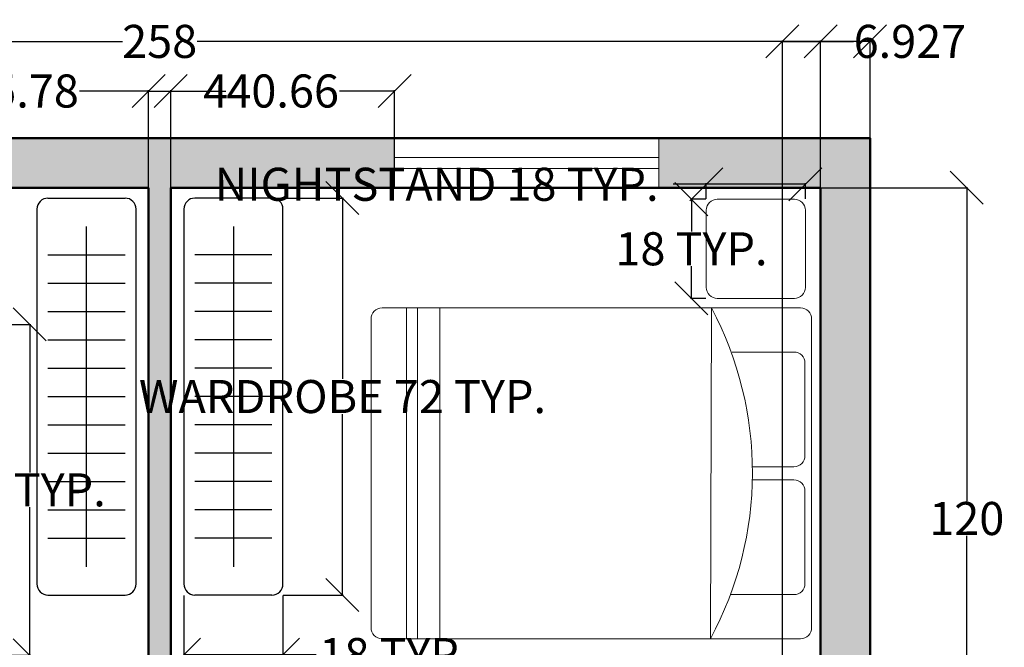
# Model space of a CAD drawing. Units: inches. Extents: x -29 to 284, y -310 to 51.
# Tile 4 of 4: x 105 to 283, y -63 to 51. Entities that reach past the tile are written whole.
import ezdxf

# ---------------------------------------------------------------- set-up
doc = ezdxf.new("R2010")
doc.units = ezdxf.units.IN
doc.header["$MEASUREMENT"] = 0
for name, color, linetype, lineweight in [('A-ANNO-DIMS', 2, 'Continuous', 18), ('A-FLOR-CASE', 9, 'Continuous', 25), ('A-FURN', 8, 'Continuous', 18), ('A-GLAZ', 4, 'Continuous', 18), ('A-WALL', 7, 'Continuous', 50)]:
    doc.layers.add(name, color=color, linetype=linetype, lineweight=lineweight)
doc.layers.add('A-WALL-PATT', color=18, linetype='Continuous', lineweight=13, true_color=0x000000)
doc.styles.get("Standard").update_dxf_attribs({"font": 'arial.ttf'})
doc.dimstyles.get("Standard").update_dxf_attribs({"dimtxt": 6, "dimasz": 6, "dimexe": 0.18, "dimexo": 0.0625, "dimgap": 0.09, "dimtad": 0, "dimtih": 1, "dimtoh": 1, "dimdec": 0, "dimzin": 0, "dimdsep": 46, "dimlunit": 4, "dimtxsty": 'Standard', "dimblk": 'OBLIQUE', "dimcen": 0.09, "dimadec": 0, "dimazin": 0, "dimtfac": 1, "dimtdec": 0, "dimtofl": 0, "dimtmove": 0, "dimatfit": 3, "dimldrblk": 'OBLIQUE', "dimfxl": 1, "dimtolj": 1, "dimtzin": 0, "dimarcsym": 0})

# ---------------------------------------------------------------- blocks, each defined once
blk = doc.blocks.new('Bed - Queen')
for p, q in [((2, 0), (58, 0)), ((10, -1.2), (26.8, -1.2)), ((33.2, -1.2), (50, -1.2)), ((0, -78), (0, -2)), ((8, -14.4), (8, -3.2)), ((28.8, -3.2), (28.8, -10.75)), ((31.2, -10.81), (31.2, -3.2)), ((52, -3.2), (52, -14.74)), ((60, -2), (60, -78)), ((0, -18.19), (60, -18.37)), ((0, -67.53), (60, -67.53)), ((0, -71.53), (60, -71.53)), ((0, -73.53), (60, -73.53)), ((58, -80), (2, -80))]:
    blk.add_line(p, q)
for centre, radius, start, end in [((2, -2), 2, 90, 180), ((58, -2), 2, 0, 90), ((10, -3.2), 2, 90, 180), ((26.8, -3.2), 2, 0, 90), ((33.2, -3.2), 2, 90, 180), ((50, -3.2), 2, 0, 90), ((29.83, -74.22), 63.48, 61.626, 118.0335), ((2, -78), 2, 180, 270), ((58, -78), 2, 270, 0)]:
    blk.add_arc(centre, radius, start, end)
blk = doc.blocks.new('WIN-48IN')
for p, q in [((0, 5.5), (48, 5.5)), ((0, 3.5), (48, 3.5))]:
    blk.add_line(p, q)
for points in [[(0, 0), (0, 9)], [(48, 9), (48, 0)]]:
    blk.add_lwpolyline(points)
blk = doc.blocks.new('WARDROBE-72IN')
for p, q in [((16, 72), (2, 72)), ((0, 70), (0, 2)), ((18, 2), (18, 70)), ((9, 66.86), (9, 5.14)), ((16, 61.71), (2, 61.71)), ((16, 56.57), (2, 56.57)), ((16, 51.43), (2, 51.43)), ((16, 46.29), (2, 46.29)), ((16, 41.14), (2, 41.14)), ((16, 36), (2, 36)), ((16, 30.86), (2, 30.86)), ((16, 25.71), (2, 25.71)), ((16, 20.57), (2, 20.57)), ((16, 15.43), (2, 15.43)), ((16, 10.29), (2, 10.29)), ((16, 0), (2, 0))]:
    blk.add_line(p, q)
for centre, start, end in [((2, 70), 90, 180), ((16, 70), 0, 90), ((2, 2), 180, 270), ((16, 2), 270, 0)]:
    blk.add_arc(centre, 2, start, end)
blk = doc.blocks.new('NIGHTSTAND-18IN')
blk.add_lwpolyline([(0, 2), (0, 16, -0.414214), (2, 18), (16, 18, -0.414214), (18, 16), (18, 2, -0.414214), (16, 0), (2, 0, -0.414214)], format="xyb", close=True)
blk = doc.blocks.new('_Oblique')
at = {"color": 0, "linetype": 'ByBlock', "lineweight": -2}
blk.add_line((-0.5, -0.5), (0.5, 0.5), dxfattribs=at)
blk = doc.blocks.new('*D23')
at = {"layer": 'A-ANNO-DIMS', "color": 0, "lineweight": -2, "transparency": 16777216}
for p, q in [((229.24, 21.07), (223.24, 21.07)), ((229.24, 18.43), (229.24, 21.25)), ((247.24, 21.07), (229.24, 21.07)), ((247.24, 18.43), (247.24, 21.25))]:
    blk.add_line(p, q, dxfattribs=at)
at = {"layer": 'Defpoints', "color": 0, "transparency": 16777216}
for p in [(229.24, 21.07), (229.24, 18.37), (247.24, 18.37)]:
    blk.add_point(p, dxfattribs=at)
at = {"layer": 'A-ANNO-DIMS', "color": 0, "lineweight": -2, "transparency": 16777216, "xscale": 6, "yscale": 6, "zscale": 6, "rotation": 180}
blk.add_blockref('_Oblique', (229.24, 21.07), dxfattribs=at)
at = {"layer": 'A-ANNO-DIMS', "color": 0, "lineweight": -2, "transparency": 16777216, "xscale": 6, "yscale": 6, "zscale": 6}
blk.add_blockref('_Oblique', (247.24, 21.07), dxfattribs=at)
at = {"layer": 'A-ANNO-DIMS', "color": 0, "transparency": 16777216, "insert": (180.28, 21.07), "char_height": 6, "attachment_point": 5}
blk.add_mtext('\\A1;NIGHTSTAND 18 TYP.', dxfattribs=at)
blk = doc.blocks.new('*D24')
at = {"layer": 'A-ANNO-DIMS', "color": 0, "lineweight": -2, "transparency": 16777216}
for p, q in [((229.17, 18.37), (226.36, 18.37)), ((226.54, 18.37), (226.54, 12.52)), ((226.54, 0.37), (226.54, 6.21)), ((229.17, 0.37), (226.36, 0.37))]:
    blk.add_line(p, q, dxfattribs=at)
at = {"layer": 'Defpoints', "color": 0, "transparency": 16777216}
for p in [(229.24, 18.37), (226.54, 0.37), (229.24, 0.37)]:
    blk.add_point(p, dxfattribs=at)
at = {"layer": 'A-ANNO-DIMS', "color": 0, "lineweight": -2, "transparency": 16777216, "xscale": 6, "yscale": 6, "zscale": 6}
for p, rotation in [((226.54, 18.37), 90), ((226.54, 0.37), 270)]:
    blk.add_blockref('_Oblique', p, dxfattribs=dict(at, rotation=rotation))
at = {"layer": 'A-ANNO-DIMS', "color": 0, "transparency": 16777216, "insert": (226.54, 9.37), "char_height": 6, "attachment_point": 5}
blk.add_mtext('\\A1;18 TYP.', dxfattribs=at)
blk = doc.blocks.new('*D26')
at = {"layer": 'A-ANNO-DIMS', "color": 0, "lineweight": -2, "transparency": 16777216}
for p, q in [((94.44, -4.36), (106.56, -4.36)), ((106.38, -4.36), (106.38, -31.2)), ((106.38, -64.36), (106.38, -37.51)), ((94.44, -64.36), (106.56, -64.36))]:
    blk.add_line(p, q, dxfattribs=at)
at = {"layer": 'Defpoints', "color": 0, "transparency": 16777216}
for p in [(94.38, -4.36), (106.38, -4.36), (94.38, -64.36)]:
    blk.add_point(p, dxfattribs=at)
at = {"layer": 'A-ANNO-DIMS', "color": 0, "lineweight": -2, "transparency": 16777216, "xscale": 6, "yscale": 6, "zscale": 6}
for p, rotation in [((106.38, -4.36), 90), ((106.38, -64.36), 270)]:
    blk.add_blockref('_Oblique', p, dxfattribs=dict(at, rotation=rotation))
at = {"layer": 'A-ANNO-DIMS', "color": 0, "transparency": 16777216, "insert": (106.38, -34.36), "char_height": 6, "attachment_point": 5}
blk.add_mtext('\\A1;60 TYP.', dxfattribs=at)
blk = doc.blocks.new('*D31')
at = {"layer": 'A-ANNO-DIMS', "color": 0, "lineweight": -2, "transparency": 16777216}
for p, q in [((152.43, 18.56), (163.35, 18.56)), ((163.17, 18.56), (163.17, -14.25)), ((163.17, -53.44), (163.17, -20.63)), ((152.43, -53.44), (163.35, -53.44))]:
    blk.add_line(p, q, dxfattribs=at)
at = {"layer": 'Defpoints', "color": 0, "transparency": 16777216}
for p in [(152.37, 18.56), (163.17, 18.56), (152.37, -53.44)]:
    blk.add_point(p, dxfattribs=at)
at = {"layer": 'A-ANNO-DIMS', "color": 0, "lineweight": -2, "transparency": 16777216, "xscale": 6, "yscale": 6, "zscale": 6}
for p, rotation in [((163.17, 18.56), 90), ((163.17, -53.44), 270)]:
    blk.add_blockref('_Oblique', p, dxfattribs=dict(at, rotation=rotation))
at = {"layer": 'A-ANNO-DIMS', "color": 0, "transparency": 16777216, "insert": (163.17, -17.44), "char_height": 6, "attachment_point": 5}
blk.add_mtext('\\A1;WARDROBE 72 TYP.', dxfattribs=at)
blk = doc.blocks.new('*D32')
at = {"layer": 'A-ANNO-DIMS', "color": 0, "lineweight": -2, "transparency": 16777216}
for p, q in [((134.37, -53.5), (134.37, -64.42)), ((152.37, -53.5), (152.37, -64.42)), ((134.37, -64.24), (152.37, -64.24)), ((152.37, -64.24), (158.37, -64.24))]:
    blk.add_line(p, q, dxfattribs=at)
at = {"layer": 'Defpoints', "color": 0, "transparency": 16777216}
for p in [(134.37, -53.44), (152.37, -53.44), (152.37, -64.24)]:
    blk.add_point(p, dxfattribs=at)
at = {"layer": 'A-ANNO-DIMS', "color": 0, "lineweight": -2, "transparency": 16777216, "xscale": 6, "yscale": 6, "zscale": 6, "rotation": 180}
blk.add_blockref('_Oblique', (134.37, -64.24), dxfattribs=at)
at = {"layer": 'A-ANNO-DIMS', "color": 0, "lineweight": -2, "transparency": 16777216, "xscale": 6, "yscale": 6, "zscale": 6}
blk.add_blockref('_Oblique', (152.37, -64.24), dxfattribs=at)
at = {"layer": 'A-ANNO-DIMS', "color": 0, "transparency": 16777216, "insert": (172.78, -64.24), "char_height": 6, "attachment_point": 5}
blk.add_mtext('\\A1;18 TYP.', dxfattribs=at)
blk = doc.blocks.new('*D45')
at = {"layer": 'A-ANNO-DIMS', "color": 0, "lineweight": -2, "transparency": 16777216}
for p, q in [((0.98, 29.5), (0.98, 47.17)), ((0.98, 46.99), (123.21, 46.99)), ((258.98, 46.99), (136.76, 46.99)), ((258.98, 29.5), (258.98, 47.17))]:
    blk.add_line(p, q, dxfattribs=at)
at = {"layer": 'Defpoints', "color": 0, "transparency": 16777216}
for p in [(258.98, 46.99), (0.98, 29.44), (258.98, 29.44)]:
    blk.add_point(p, dxfattribs=at)
at = {"layer": 'A-ANNO-DIMS', "color": 0, "lineweight": -2, "transparency": 16777216, "xscale": 6, "yscale": 6, "zscale": 6, "rotation": 180}
blk.add_blockref('_Oblique', (0.98, 46.99), dxfattribs=at)
at = {"layer": 'A-ANNO-DIMS', "color": 0, "lineweight": -2, "transparency": 16777216, "xscale": 6, "yscale": 6, "zscale": 6}
blk.add_blockref('_Oblique', (258.98, 46.99), dxfattribs=at)
at = {"layer": 'A-ANNO-DIMS', "color": 0, "transparency": 16777216, "insert": (129.98, 46.99), "char_height": 6, "attachment_point": 5}
blk.add_mtext('\\A1;258', dxfattribs=at)
blk = doc.blocks.new('*D48')
at = {"layer": 'A-ANNO-DIMS', "color": 0, "lineweight": -2, "transparency": 16777216}
for p, q in [((82.2, 20.5), (82.2, 38.17)), ((82.2, 37.99), (94.75, 37.99)), ((127.98, 37.99), (115.43, 37.99)), ((127.98, 20.5), (127.98, 38.17))]:
    blk.add_line(p, q, dxfattribs=at)
at = {"layer": 'Defpoints', "color": 0, "transparency": 16777216}
for p in [(127.98, 37.99), (82.2, 20.44), (127.98, 20.44)]:
    blk.add_point(p, dxfattribs=at)
at = {"layer": 'A-ANNO-DIMS', "color": 0, "lineweight": -2, "transparency": 16777216, "xscale": 6, "yscale": 6, "zscale": 6, "rotation": 180}
blk.add_blockref('_Oblique', (82.2, 37.99), dxfattribs=at)
at = {"layer": 'A-ANNO-DIMS', "color": 0, "lineweight": -2, "transparency": 16777216, "xscale": 6, "yscale": 6, "zscale": 6}
blk.add_blockref('_Oblique', (127.98, 37.99), dxfattribs=at)
at = {"layer": 'A-ANNO-DIMS', "color": 0, "transparency": 16777216, "insert": (105.09, 37.99), "char_height": 6, "attachment_point": 5}
blk.add_mtext('\\A1;45.78', dxfattribs=at)
blk = doc.blocks.new('*D49')
at = {"layer": 'A-ANNO-DIMS', "color": 0, "lineweight": -2, "transparency": 16777216}
for p, q in [((127.98, 20.5), (127.98, 38.17)), ((127.98, 37.99), (131.98, 37.99)), ((131.98, 20.5), (131.98, 38.17)), ((131.98, 37.99), (137.98, 37.99))]:
    blk.add_line(p, q, dxfattribs=at)
at = {"layer": 'Defpoints', "color": 0, "transparency": 16777216}
for p in [(131.98, 37.99), (127.98, 20.44), (131.98, 20.44)]:
    blk.add_point(p, dxfattribs=at)
at = {"layer": 'A-ANNO-DIMS', "color": 0, "lineweight": -2, "transparency": 16777216, "xscale": 6, "yscale": 6, "zscale": 6, "rotation": 180}
blk.add_blockref('_Oblique', (127.98, 37.99), dxfattribs=at)
at = {"layer": 'A-ANNO-DIMS', "color": 0, "lineweight": -2, "transparency": 16777216, "xscale": 6, "yscale": 6, "zscale": 6}
blk.add_blockref('_Oblique', (131.98, 37.99), dxfattribs=at)
at = {"layer": 'A-ANNO-DIMS', "color": 0, "transparency": 16777216, "insert": (140.15, 37.99), "char_height": 6, "attachment_point": 5}
blk.add_mtext('\\A1;4', dxfattribs=at)
blk = doc.blocks.new('*D50')
at = {"layer": 'A-ANNO-DIMS', "color": 0, "lineweight": -2, "transparency": 16777216}
for p, q in [((131.98, 20.5), (131.98, 38.17)), ((131.98, 37.99), (141.98, 37.99)), ((172.64, 37.99), (162.64, 37.99)), ((172.64, 20.5), (172.64, 38.17))]:
    blk.add_line(p, q, dxfattribs=at)
at = {"layer": 'Defpoints', "color": 0, "transparency": 16777216}
for p in [(172.64, 37.99), (131.98, 20.44), (172.64, 20.44)]:
    blk.add_point(p, dxfattribs=at)
at = {"layer": 'A-ANNO-DIMS', "color": 0, "lineweight": -2, "transparency": 16777216, "xscale": 6, "yscale": 6, "zscale": 6, "rotation": 180}
blk.add_blockref('_Oblique', (131.98, 37.99), dxfattribs=at)
at = {"layer": 'A-ANNO-DIMS', "color": 0, "lineweight": -2, "transparency": 16777216, "xscale": 6, "yscale": 6, "zscale": 6}
blk.add_blockref('_Oblique', (172.64, 37.99), dxfattribs=at)
at = {"layer": 'A-ANNO-DIMS', "color": 0, "transparency": 16777216, "insert": (152.31, 37.99), "char_height": 6, "attachment_point": 5}
blk.add_mtext('\\A1;40.66', dxfattribs=at)
blk = doc.blocks.new('*D51')
at = {"layer": 'A-ANNO-DIMS', "color": 0, "lineweight": -2, "transparency": 16777216}
for p, q in [((250.04, 20.44), (276.71, 20.44)), ((276.53, 20.44), (276.53, -36.41)), ((276.53, -99.56), (276.53, -42.72)), ((250.04, -99.56), (276.71, -99.56))]:
    blk.add_line(p, q, dxfattribs=at)
at = {"layer": 'Defpoints', "color": 0, "transparency": 16777216}
for p in [(249.98, 20.44), (249.98, -99.56), (276.53, -99.56)]:
    blk.add_point(p, dxfattribs=at)
at = {"layer": 'A-ANNO-DIMS', "color": 0, "lineweight": -2, "transparency": 16777216, "xscale": 6, "yscale": 6, "zscale": 6}
for p, rotation in [((276.53, 20.44), 90), ((276.53, -99.56), 270)]:
    blk.add_blockref('_Oblique', p, dxfattribs=dict(at, rotation=rotation))
at = {"layer": 'A-ANNO-DIMS', "color": 0, "transparency": 16777216, "insert": (276.53, -39.56), "char_height": 6, "attachment_point": 5}
blk.add_mtext('\\A1;120', dxfattribs=at)
blk = doc.blocks.new('*D68')
at = {"layer": 'A-ANNO-DIMS', "color": 0, "lineweight": -2, "transparency": 16777216}
for p, q in [((243.05, -108.33), (243.05, 47.17)), ((243.05, 46.99), (249.98, 46.99)), ((249.98, -103.5), (249.98, 47.17)), ((249.98, 46.99), (255.98, 46.99))]:
    blk.add_line(p, q, dxfattribs=at)
at = {"layer": 'Defpoints', "color": 0, "transparency": 16777216}
for p in [(249.98, 46.99), (249.98, -103.56), (243.05, -108.39)]:
    blk.add_point(p, dxfattribs=at)
at = {"layer": 'A-ANNO-DIMS', "color": 0, "lineweight": -2, "transparency": 16777216, "xscale": 6, "yscale": 6, "zscale": 6, "rotation": 180}
blk.add_blockref('_Oblique', (243.05, 46.99), dxfattribs=at)
at = {"layer": 'A-ANNO-DIMS', "color": 0, "lineweight": -2, "transparency": 16777216, "xscale": 6, "yscale": 6, "zscale": 6}
blk.add_blockref('_Oblique', (249.98, 46.99), dxfattribs=at)
at = {"layer": 'A-ANNO-DIMS', "color": 0, "transparency": 16777216, "insert": (266.21, 46.99), "char_height": 6, "attachment_point": 5}
blk.add_mtext('\\A1;6.927', dxfattribs=at)

msp = doc.modelspace()

# ---------------------------------------------------------------- hatches: boundary and pattern name
at = {"layer": 'A-WALL-PATT'}
h = msp.add_hatch(color=256, dxfattribs=at)
h.dxf.hatch_style = 1
h.paths.add_polyline_path([(172.6409, 20.4365), (172.6409, 29.4365), (82.1984, 29.4365), (82.1984, 20.4365), (127.9809, 20.4365), (127.9809, -99.5635), (121.9809, -99.5635), (121.9809, -103.5635), (127.9809, -103.5635), (137.9809, -103.5635), (137.9809, -99.5635), (131.9809, -99.5635), (131.9809, 20.4365)])
h = msp.add_hatch(color=256, dxfattribs=at)
h.dxf.hatch_style = 1
h.paths.add_polyline_path([(249.9809, 20.4365), (249.9809, -99.5635), (167.9809, -99.5635), (167.9809, -103.5635), (249.9809, -103.5635), (249.9809, -138.6614), (258.9809, -138.6614), (258.9809, 29.4365), (220.6409, 29.4365), (220.6409, 20.4365)])

# ---------------------------------------------------------------- linework, layer by layer
at = {"layer": 'A-WALL'}
for p, q in [((9.9809, 20.4365), (127.9809, 20.4365)), ((127.9809, -99.5635), (127.9809, 20.4365)), ((131.9809, -99.5635), (131.9809, 20.4365)), ((131.9809, 20.4365), (249.9809, 20.4365)), ((249.9809, 20.4365), (249.9809, -99.5635))]:
    msp.add_line(p, q, dxfattribs=at)
msp.add_lwpolyline([(99.9809, -288.5635), (0.9809, -288.5635), (0.9809, 29.4365), (258.9809, 29.4365), (258.9809, -288.5635), (135.9809, -288.5635)], dxfattribs=at)

# ---------------------------------------------------------------- block references
at = {"layer": 'A-FLOR-CASE', "rotation": 180}
msp.add_blockref('WARDROBE-72IN', (125.6986, 18.5591), dxfattribs=at)
at = {"layer": 'A-FLOR-CASE'}
msp.add_blockref('WARDROBE-72IN', (134.369, -53.44), dxfattribs=at)
at = {"layer": 'A-FURN'}
for name, p, rotation in [('NIGHTSTAND-18IN', (247.2349, 18.3659), 180), ('Bed - Queen', (248.3535, -1.3681), 270)]:
    msp.add_blockref(name, p, dxfattribs=dict(at, rotation=rotation))
at = {"layer": 'A-GLAZ'}
msp.add_blockref('WIN-48IN', (172.641, 20.437), dxfattribs=at)

# ---------------------------------------------------------------- dimensions: what is measured, and where the dimension line sits
at = {"layer": 'A-ANNO-DIMS'}
for base, p1, p2, override, picture, middle in [((258.9809, 46.9865), (0.9809, 29.4365), (258.9809, 29.4365), {"dimdec": 0, "dimlfac": 1, "dimrnd": 0, "dimzin": 0, "dimdsep": 46, "dimlunit": 2}, '*D45', (129.9809, 46.9865)), ((249.9809, 46.9865), (243.054, -108.39), (249.9809, -103.5635), {"dimdec": 3, "dimlfac": 1, "dimrnd": 0, "dimzin": 0, "dimdsep": 46, "dimlunit": 2}, '*D68', (266.2108, 46.9865)), ((131.9809, 37.9865), (127.9809, 20.4365), (131.9809, 20.4365), {"dimdec": 0, "dimlfac": 1, "dimrnd": 0, "dimzin": 0, "dimdsep": 46, "dimlunit": 2}, '*D49', (140.146, 37.9865)), ((172.6409, 37.9865), (131.9809, 20.4365), (172.6409, 20.4365), {"dimdec": 2, "dimlfac": 1, "dimrnd": 0, "dimzin": 0, "dimdsep": 46, "dimlunit": 2}, '*D50', (152.3109, 37.9865))]:
    dim = msp.add_linear_dim(base=base, p1=p1, p2=p2, dimstyle='Standard', override=override, dxfattribs=at)
    dim.commit()
    dim.dimension.update_dxf_attribs({"geometry": picture, "text_midpoint": middle})
for base, p1, p2, angle, override, picture, middle in [((127.9809, 37.9865), (82.1984, 20.4365), (127.9809, 20.4365), 0, {"dimdec": 2, "dimlfac": 1, "dimrnd": 0, "dimzin": 0, "dimdsep": 46, "dimlunit": 2}, '*D48', (105.0897, 37.9865)), ((276.5309, -99.5635), (249.9809, 20.4365), (249.9809, -99.5635), 90, {"dimdec": 0, "dimlfac": 1, "dimrnd": 0, "dimzin": 0, "dimdsep": 46, "dimlunit": 2}, '*D51', (276.5309, -39.5635))]:
    dim = msp.add_linear_dim(base=base, p1=p1, p2=p2, angle=angle, dimstyle='Standard', override=override, dxfattribs=at)
    dim.commit()
    dim.dimension.update_dxf_attribs({"geometry": picture, "text_midpoint": middle})
for base, p1, p2, angle, text, picture, middle in [((229.2351, 21.0664), (247.2351, 18.3664), (229.2351, 18.3664), 180, 'NIGHTSTAND <> TYP.', '*D23', (180.2815, 21.0664)), ((163.1688, 18.5596), (152.3688, -53.4404), (152.3688, 18.5596), 90, 'WARDROBE <> TYP.', '*D31', (163.1688, -17.4404)), ((226.5351, 0.3664), (229.2351, 18.3664), (229.2351, 0.3664), 270, '<> TYP.', '*D24', (226.5351, 9.3664)), ((106.3804, -4.3576), (94.3804, -64.3576), (94.3804, -4.3576), 90, '<> TYP.', '*D26', (106.3804, -34.3576))]:
    dim = msp.add_linear_dim(base=base, p1=p1, p2=p2, angle=angle, text=text, dimstyle='Standard', override={"dimdec": 0, "dimlfac": 1, "dimrnd": 0, "dimzin": 0, "dimdsep": 46, "dimlunit": 2}, dxfattribs=at)
    dim.commit()
    dim.dimension.update_dxf_attribs({"geometry": picture, "text_midpoint": middle})
dim = msp.add_linear_dim(base=(152.3688, -64.2404), p1=(134.3688, -53.4404), p2=(152.3688, -53.4404), text='<> TYP.', dimstyle='Standard', override={"dimdec": 0, "dimlfac": 1, "dimrnd": 0, "dimzin": 0, "dimdsep": 46, "dimlunit": 2}, dxfattribs=at)
dim.commit()
dim.dimension.update_dxf_attribs({"geometry": '*D32', "text_midpoint": (172.7794, -64.2404)})

doc.saveas('drawing.dxf')
